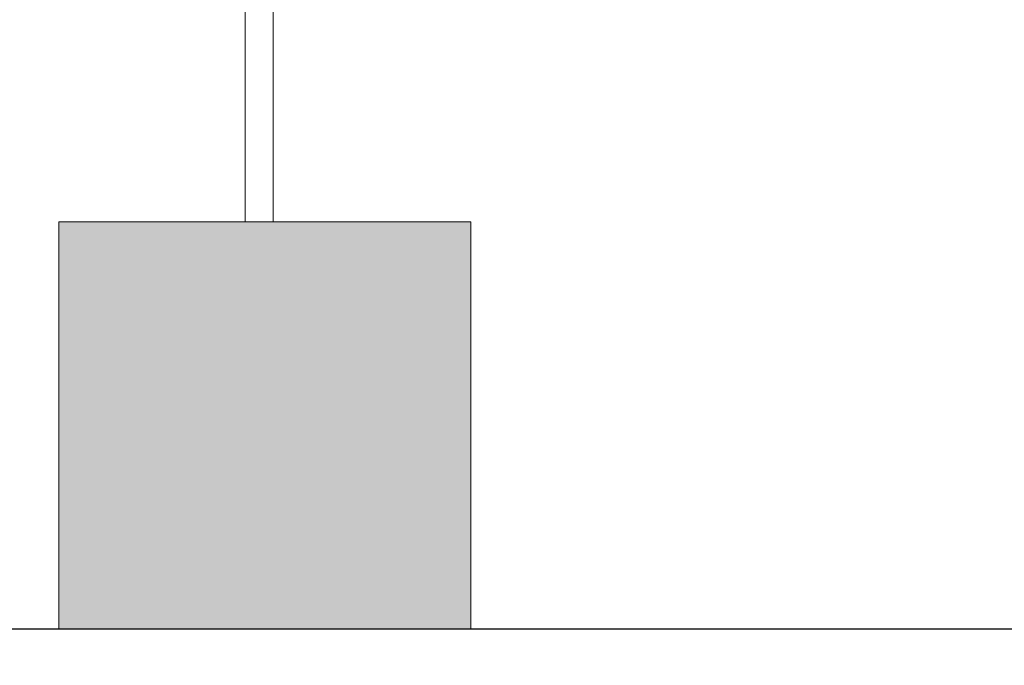
# Model space of a CAD drawing. Units: millimetres. Extents: x 7894 to 8038, y 6851 to 6951.
# Tile 29 of 49: x 7958.696 to 7962.874, y 6922.974 to 6925.713. Entities that reach past the tile are written whole.
import ezdxf

# ---------------------------------------------------------------- set-up
doc = ezdxf.new("R2010")
doc.units = ezdxf.units.MM
for name, color, linetype, lineweight in [('A-ANNO-DIMS', 2, 'Continuous', 18), ('A-FURN-ACCS', 8, 'Continuous', 13), ('A-FURN-SHLF', 7, 'Continuous', 30)]:
    doc.layers.add(name, color=color, linetype=linetype, lineweight=lineweight)
doc.layers.add('A-FURN-ACCS-PATT', color=116, linetype='Continuous', lineweight=9, true_color=0x136734)
doc.styles.get("Standard").update_dxf_attribs({"font": 'arial.ttf'})
doc.dimstyles.new('ISO-25', dxfattribs={"dimtxt": 1, "dimasz": 1, "dimexe": 1.25, "dimexo": 0.625, "dimtad": 1, "dimdec": 0, "dimlunit": 4, "dimtxsty": 'Standard', "dimcen": 2.5, "dimclrt": 1, "dimadec": 0, "dimazin": 0, "dimtfac": 1, "dimtdec": 0, "dimtmove": 0, "dimatfit": 3, "dimfxl": 1, "dimarcsym": 0})

# ---------------------------------------------------------------- blocks, each defined once
blk = doc.blocks.new('DISPLAY-LEAF-FINIAL-Z2_152')
for p, q in [((0.7416, 0, 2.1518), (0.7416, 1.0372, 2.1518)), ((0.8605, 0, 2.1518), (0.8605, 0.9923, 2.1518))]:
    blk.add_line(p, q)
blk = doc.blocks.new('*D23')
at = {"layer": 'A-ANNO-DIMS', "color": 0, "lineweight": -2, "transparency": 16777216}
for p, q in [((7940.0888, 6907.098), (7940.0888, 6947.7928)), ((7971.9356, 6928.989), (7971.9356, 6947.7928)), ((7941.0888, 6946.5428), (7970.9356, 6946.5428))]:
    blk.add_line(p, q, dxfattribs=at)
at = {"layer": 'A-ANNO-DIMS', "color": 0, "transparency": 16777216}
for points in [[(7941.0888, 6946.7095), (7941.0888, 6946.3762), (7940.0888, 6946.5428)], [(7970.9356, 6946.7095), (7970.9356, 6946.3762), (7971.9356, 6946.5428)]]:
    blk.add_solid(points, dxfattribs=at)
at = {"layer": 'Defpoints', "color": 0, "transparency": 16777216}
for p in [(7971.9356, 6946.5428), (7971.9356, 6928.364), (7940.0888, 6906.473)]:
    blk.add_point(p, dxfattribs=at)
at = {"layer": 'A-ANNO-DIMS', "color": 1, "transparency": 16777216, "insert": (7956.0122, 6947.6784), "char_height": 1, "attachment_point": 5}
blk.add_mtext('2\'-8"', dxfattribs=at)
blk = doc.blocks.new('*D28')
at = {"layer": 'A-ANNO-DIMS', "color": 0, "lineweight": -2, "transparency": 16777216}
for p, q in [((7960.8854, 6936.8804), (7975.2272, 6936.8804)), ((7973.9772, 6935.8804), (7973.9772, 6923.6283)), ((7971.8421, 6922.6283), (7975.2272, 6922.6283))]:
    blk.add_line(p, q, dxfattribs=at)
at = {"layer": 'A-ANNO-DIMS', "color": 0, "transparency": 16777216}
for points in [[(7973.8105, 6935.8804), (7974.1439, 6935.8804), (7973.9772, 6936.8804)], [(7973.8105, 6923.6283), (7974.1439, 6923.6283), (7973.9772, 6922.6283)]]:
    blk.add_solid(points, dxfattribs=at)
at = {"layer": 'Defpoints', "color": 0, "transparency": 16777216}
for p in [(7960.2604, 6936.8804), (7971.2171, 6922.6283), (7973.9772, 6922.6283)]:
    blk.add_point(p, dxfattribs=at)
at = {"layer": 'A-ANNO-DIMS', "color": 1, "transparency": 16777216, "insert": (7972.8351, 6929.7543), "char_height": 1, "attachment_point": 5, "rotation": 90}
blk.add_mtext('1\'-2 1/2"', dxfattribs=at)
blk = doc.blocks.new('*D31')
at = {"layer": 'A-ANNO-DIMS', "color": 0, "lineweight": -2, "transparency": 16777216}
for p, q in [((7973.9772, 6921.7198), (7973.9772, 6926.628)), ((7949.8107, 6920.7198), (7975.2272, 6920.7198)), ((7973.9772, 6918.7198), (7973.9772, 6920.7198)), ((7950.9654, 6918.7198), (7975.2272, 6918.7198)), ((7973.9772, 6917.7198), (7973.9772, 6916.7198))]:
    blk.add_line(p, q, dxfattribs=at)
at = {"layer": 'A-ANNO-DIMS', "color": 0, "transparency": 16777216}
for points in [[(7973.8105, 6921.7198), (7974.1439, 6921.7198), (7973.9772, 6920.7198)], [(7973.8105, 6917.7198), (7974.1439, 6917.7198), (7973.9772, 6918.7198)]]:
    blk.add_solid(points, dxfattribs=at)
at = {"layer": 'Defpoints', "color": 0, "transparency": 16777216}
for p in [(7949.1857, 6920.7198), (7973.9772, 6920.7198), (7950.3404, 6918.7198)]:
    blk.add_point(p, dxfattribs=at)
at = {"layer": 'A-ANNO-DIMS', "color": 1, "transparency": 16777216, "insert": (7972.8416, 6924.6739), "char_height": 1, "attachment_point": 5, "rotation": 90}
blk.add_mtext('0\'-2"', dxfattribs=at)

msp = doc.modelspace()

# ---------------------------------------------------------------- hatches: boundary and pattern name
at = {"layer": 'A-FURN-ACCS-PATT'}
h = msp.add_hatch(color=256, dxfattribs=at)
h.dxf.hatch_style = 1
h.paths.add_polyline_path([(7947.5161, 6931.8853), (7946.6774, 6931.8853), (7946.5585, 6931.8853), (7945.7683, 6931.8853), (7945.7683, 6930.1581), (7947.5161, 6930.1581)])
h.paths.add_polyline_path([(7947.4851, 6922.447), (7946.6464, 6922.447), (7946.5276, 6922.447), (7945.7373, 6922.447), (7945.7373, 6920.7198), (7947.4851, 6920.7198)])
h.paths.add_polyline_path([(7968.0212, 6935.881), (7967.1825, 6935.881), (7967.0637, 6935.881), (7966.2734, 6935.881), (7966.2734, 6934.1538), (7968.0212, 6934.1538)])
h.paths.add_polyline_path([(7960.6099, 6924.8555), (7959.7712, 6924.8555), (7959.6523, 6924.8555), (7958.862, 6924.8555), (7958.862, 6923.1283), (7960.6099, 6923.1283)])
h.paths.add_polyline_path([(7964.717, 6924.8555), (7963.8783, 6924.8555), (7963.7594, 6924.8555), (7962.9691, 6924.8555), (7962.9691, 6923.1283), (7964.717, 6923.1283)])
h.paths.add_polyline_path([(7971.0698, 6924.8555), (7970.2311, 6924.8555), (7970.1123, 6924.8555), (7969.322, 6924.8555), (7969.322, 6923.1283), (7971.0698, 6923.1283)])
h.paths.add_polyline_path([(7958.5294, 6908.7006), (7957.6907, 6908.7006), (7957.5718, 6908.7006), (7956.7815, 6908.7006), (7956.7815, 6906.9734), (7958.5294, 6906.9734)])

# ---------------------------------------------------------------- linework, layer by layer
at = {"layer": 'A-FURN-ACCS'}
for p, q in [((7958.862, 6923.1283, 2.1518), (7958.862, 6924.8555, 2.1518)), ((7958.862, 6924.8555, 2.1518), (7959.6523, 6924.8555, 2.1518)), ((7959.7712, 6924.8555, 2.1518), (7959.6523, 6924.8555, 2.1518)), ((7959.7712, 6924.8555, 2.1518), (7960.6099, 6924.8555, 2.1518)), ((7960.6099, 6923.1283, 2.1518), (7960.6099, 6924.8555, 2.1518))]:
    msp.add_line(p, q, dxfattribs=at)
at = {"layer": 'A-FURN-SHLF'}
msp.add_line((7953.9136, 6923.1283, -7), (7971.2171, 6923.1283, -7), dxfattribs=at)

# ---------------------------------------------------------------- block references
at = {"layer": 'A-FURN-ACCS'}
msp.add_blockref('DISPLAY-LEAF-FINIAL-Z2_152', (7958.9107, 6924.8555), dxfattribs=at)

# ---------------------------------------------------------------- dimensions: what is measured, and where the dimension line sits
at = {"layer": 'A-ANNO-DIMS'}
dim = msp.add_linear_dim(base=(7971.9356, 6946.5428), p1=(7940.0888, 6906.473), p2=(7971.9356, 6928.364), dimstyle='ISO-25', override={"dimdec": 1, "dimlfac": 1, "dimrnd": 0, "dimzin": 1, "dimdsep": 46, "dimlunit": 4, "dimfrac": 2}, dxfattribs=at)
dim.commit()
dim.dimension.update_dxf_attribs({"geometry": '*D23', "text_midpoint": (7956.0122, 6947.6784)})
for base, p1, p2, picture, middle in [((7973.9772, 6922.6283), (7960.2604, 6936.8804), (7971.2171, 6922.6283), '*D28', (7972.8351, 6929.7543)), ((7973.9772, 6920.7198), (7950.3404, 6918.7198), (7949.1857, 6920.7198), '*D31', (7972.8416, 6924.6739))]:
    dim = msp.add_linear_dim(base=base, p1=p1, p2=p2, angle=90, dimstyle='ISO-25', override={"dimdec": 1, "dimlfac": 1, "dimrnd": 0, "dimzin": 1, "dimdsep": 46, "dimlunit": 4, "dimfrac": 2}, dxfattribs=at)
    dim.commit()
    dim.dimension.update_dxf_attribs({"geometry": picture, "text_midpoint": middle})

doc.saveas('drawing.dxf')
